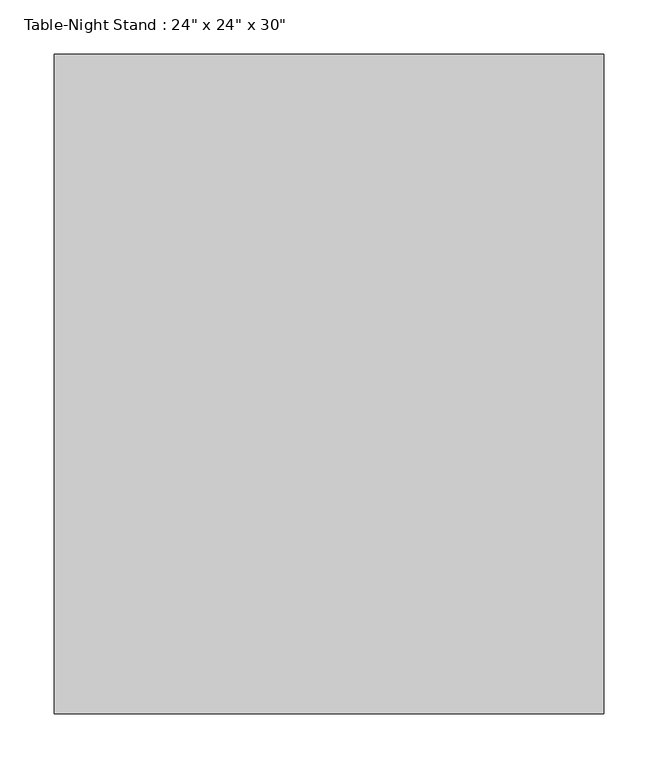
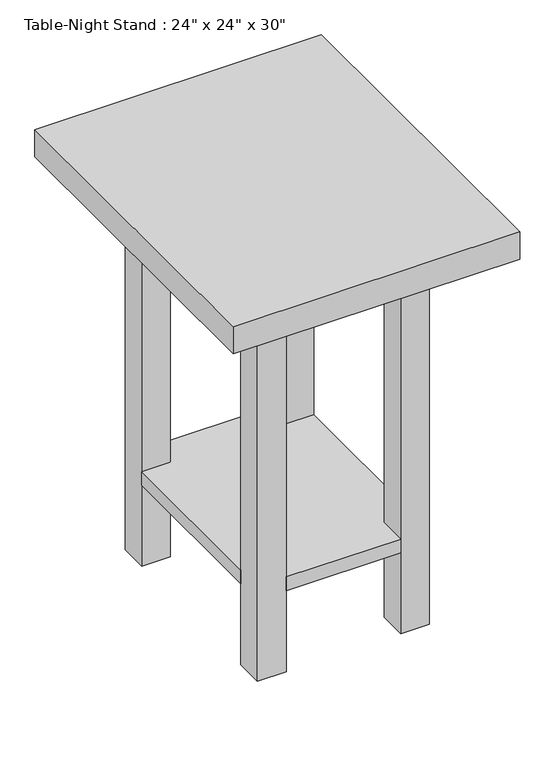
"""IFC4 building model written with IfcOpenShell, lengths in millimetres: furniture geometry."""

from ifc_helpers import new_model, si_unit, frame, origin, origin_with_axes, place, context, project, spatial, polyline, outline, extrude, source, transform, mapped, element, save


def furniture_a4b90d56(model_context):
    return source(origin(), model_context, "Body", "SweptSolid", [
        extrude(outline(polyline([(156.1336303, 508.0), (359.3336303, 508.0), (359.3336303, 457.2), (410.1336303, 457.2), (410.1336303, 152.4), (359.3336303, 152.4), (359.3336303, 101.6), (156.1336303, 101.6), (156.1336303, 152.4), (105.3336303, 152.4), (105.3336303, 457.2), (156.1336303, 457.2), (156.1336303, 508.0)])), frame((0.0, 0.0, 152.4), z_axis=(0.0, 0.0, 1.0), x_axis=(1.0, 0.0, 0.0)), (0.0, 0.0, 1.0), 25.4),
        extrude(outline(polyline([(156.1336303, 508.0), (156.1336303, 457.2), (105.3336303, 457.2), (105.3336303, 508.0), (156.1336303, 508.0)])), origin_with_axes(), (0.0, 0.0, 1.0), 711.2),
        extrude(outline(polyline([(156.1336303, 152.4), (156.1336303, 101.6), (105.3336303, 101.6), (105.3336303, 152.4), (156.1336303, 152.4)])), origin_with_axes(), (0.0, 0.0, 1.0), 711.2),
        extrude(outline(polyline([(410.1336303, 508.0), (410.1336303, 457.2), (359.3336303, 457.2), (359.3336303, 508.0), (410.1336303, 508.0)])), origin_with_axes(), (0.0, 0.0, 1.0), 711.2),
        extrude(outline(polyline([(410.1336303, 152.4), (410.1336303, 101.6), (359.3336303, 101.6), (359.3336303, 152.4), (410.1336303, 152.4)])), origin_with_axes(), (0.0, 0.0, 1.0), 711.2),
        extrude(outline(polyline([(511.7336303, 0.0), (3.7336303, 0.0), (3.7336303, 609.6), (511.7336303, 609.6), (511.7336303, 0.0)])), frame((0.0, 0.0, 711.2), z_axis=(0.0, 0.0, 1.0), x_axis=(1.0, 0.0, 0.0)), (0.0, 0.0, 1.0), 50.8),
    ])


if __name__ == "__main__":
    model = new_model("IFC4")
    model_context = context("Model", 3, world=origin())
    ifc_project = project(units=[si_unit("LENGTHUNIT", "METRE", prefix="MILLI")], contexts=[model_context])
    site = spatial("IfcSite", under=ifc_project)
    building = spatial("IfcBuilding", under=site)
    placement = place(None, origin())
    furniture_shape = furniture_a4b90d56(model_context)
    element("IfcFurniture", 1, ObjectType="Table-Night Stand : 24\" x 24\" x 30\"", at=placement, inside=building, context=model_context, shape_type="MappedRepresentation", body=[
        mapped(furniture_shape, transform((0.0, 0.0, 0.0), x_axis=(1.0, 0.0, 0.0), y_axis=(0.0, 1.0, 0.0), z_axis=(0.0, 0.0, 1.0))),
    ])
    save(model, "model.ifc")

# Revit data of these elements
# Type "Table-Night Stand : 24\" x 24\" x 30\""
#   Assembly Code = "E2020200"
#   Depth = 2' - 0"
#   Height = 2' - 6"
#   Width = 1' - 8"
#   Base Material = Birch
#   Top Material = Laminate, Ivory, Matte
#   Default Elevation = 0
# Element 1 (IfcFurniture, "Table-Night Stand : 24\" x 24\" x 30\"")
#   Materials on its faces: "Birch", "Laminate, Ivory, Matte"
# Materials
#   "Birch": class "Wood", colour RGB 224 178 126, transparency 0, Description = "Betula Alleghaniensis", Cost = 0
#   "Laminate, Ivory, Matte": class "Plastic", colour RGB 247 247 239, transparency 0, Description = "Plastic Laminate - Ivory, Matte", Cost = 0
